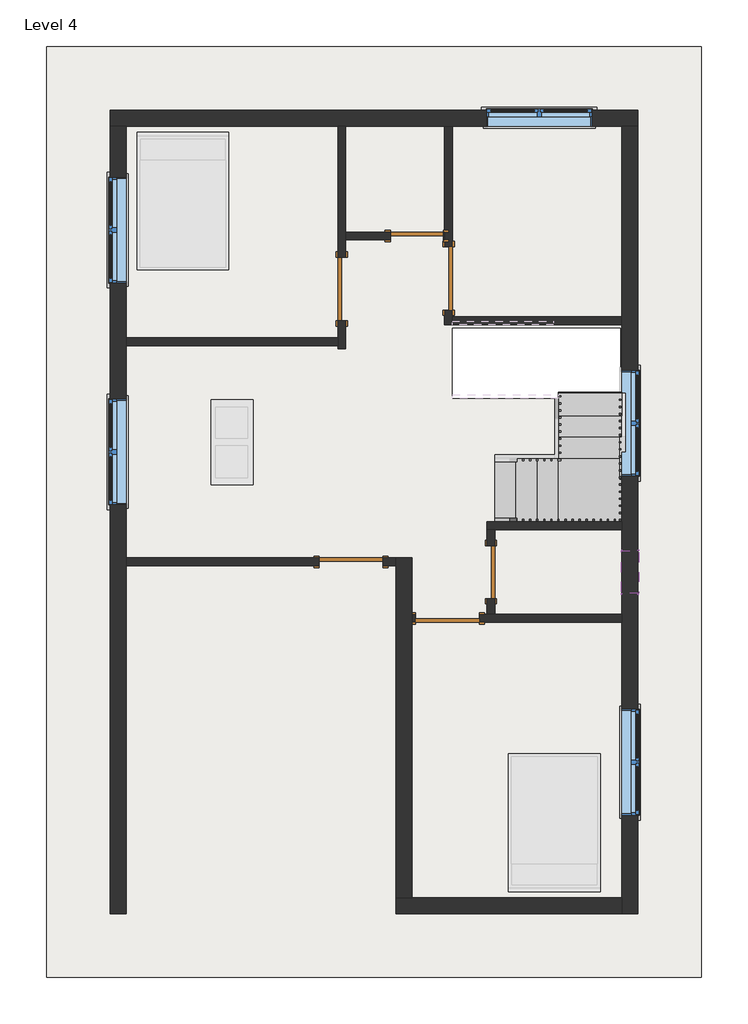
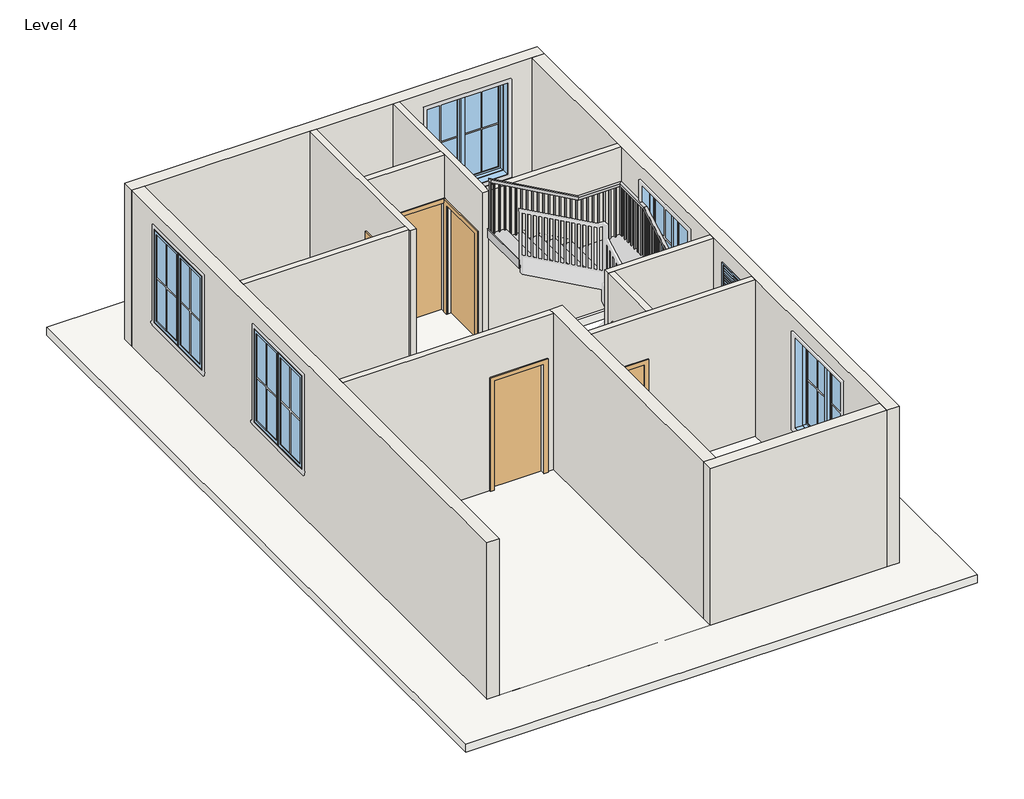
# One storey, part 1 of 2: 14 walls, 6 doors, 6 windows, 1 railing, 1 roof, 1 slab, 1 stair flight.
"""IFC4 building model written with IfcOpenShell, lengths in millimetres."""

from ifc_helpers import new_model, si_unit, frame, origin, place, context, project, spatial, polyline, outline, extrude, faceted_brep, transform, mapped, element, save
from components import door_214872d5, door_78caadf7, single_flush_door_3_e5f9f3c4, single_flush_door_3_305aa2a5, stair_flight_961aca31, window_casement_double_win_5_f93960c7, window_f2d8fef0

model = new_model("IFC4")

# Units and contexts
model_context = context("Model", 3, world=origin())
ifc_project = project(units=[si_unit("LENGTHUNIT", "METRE", prefix="MILLI")], contexts=[model_context])

# Site, building, storey
site = spatial("IfcSite", under=ifc_project)
building = spatial("IfcBuilding", under=site)
storey = spatial("IfcBuildingStorey", under=building, Name="Level 4", Elevation=6400.8)

# Doors
placement = place(None, origin())
door_shape = door_214872d5(model_context)
element("IfcDoor", 1, ObjectType="Single-Flush : DOOR 2'6\"", at=placement, inside=storey, context=model_context, shape_type="MappedRepresentation", body=[
    mapped(door_shape, transform((-185.4325206, 3926.3629493, 6400.8), x_axis=(1.0, 0.0, 0.0), y_axis=(0.0, 1.0, 0.0), z_axis=(0.0, 0.0, 1.0))),
])
door_2_shape = door_78caadf7(model_context)
element("IfcDoor", 2, ObjectType="Single-Flush : DOOR 2'6\"", at=placement, inside=storey, context=model_context, shape_type="MappedRepresentation", body=[
    mapped(door_2_shape, transform((881.3674794, -905.9870507, 6400.8), x_axis=(0.0, 1.0, 0.0), y_axis=(-1.0, 0.0, 0.0), z_axis=(0.0, 0.0, 1.0))),
])
single_flush_door_3_shape = single_flush_door_3_e5f9f3c4(model_context)
element("IfcDoor", 3, ObjectType="Single-Flush : DOOR 3'", at=placement, inside=storey, context=model_context, shape_type="MappedRepresentation", body=[
    mapped(single_flush_door_3_shape, transform((271.7674794, 3316.7629493, 6400.8), x_axis=(0.0, -1.0, 0.0), y_axis=(1.0, 0.0, 0.0), z_axis=(0.0, 0.0, 1.0))),
])
element("IfcDoor", 4, ObjectType="Single-Flush : DOOR 3'", at=placement, inside=storey, context=model_context, shape_type="MappedRepresentation", body=[
    mapped(single_flush_door_3_shape, transform((255.8924794, -1572.7370507, 6400.8), x_axis=(-1.0, 0.0, 0.0), y_axis=(0.0, -1.0, 0.0), z_axis=(0.0, 0.0, 1.0))),
])
single_flush_door_3_2_shape = single_flush_door_3_305aa2a5(model_context)
element("IfcDoor", 5, ObjectType="Single-Flush : DOOR 3'", at=placement, inside=storey, context=model_context, shape_type="MappedRepresentation", body=[
    mapped(single_flush_door_3_2_shape, transform((-1264.9325206, 3164.3629493, 6400.8), x_axis=(0.0, -1.0, 0.0), y_axis=(1.0, 0.0, 0.0), z_axis=(0.0, 0.0, 1.0))),
])
element("IfcDoor", 6, ObjectType="Single-Flush : DOOR 3'6\"", at=placement, inside=storey, context=model_context, shape_type="MappedRepresentation", body=[
    mapped(single_flush_door_3_shape, transform((-1131.5825206, -759.9370507, 6400.8), x_axis=(1.0, 0.0, 0.0), y_axis=(0.0, 1.0, 0.0), z_axis=(0.0, 0.0, 1.0))),
])

# Railing
element("IfcRailing", 7, ObjectType="Handrail - Rectangular", at=placement, inside=storey, context=model_context, shape_type="SolidModel", body=[
    faceted_brep([(938.5174794, -131.2870507, 7484.5333333), (938.5174794, -131.2870507, 7426.420221), (938.5174794, -182.0870507, 7426.420221), (938.5174794, -182.0870507, 7484.5333333), (2005.3174794, -131.2870507, 8077.2), (2018.4810817, -131.2870507, 8026.4), (2018.4810817, -182.0870507, 8026.4), (2005.3174794, -182.0870507, 8077.2), (2716.5174794, -131.2870507, 8077.2), (2716.5174794, -131.2870507, 8026.4), (2767.3174794, -182.0870507, 8026.4), (2767.3174794, -182.0870507, 8077.2), (2716.5174794, 579.9129493, 8077.2), (2716.5174794, 593.0765516, 8026.4), (2767.3174794, 593.0765516, 8026.4), (2767.3174794, 579.9129493, 8077.2), (2716.5174794, 1843.5629493, 8779.2277778), (2716.5174794, 1856.7265516, 8728.4277778), (2767.3174794, 1856.7265516, 8728.4277778), (2767.3174794, 1843.5629493, 8779.2277778), (2716.5174794, 2599.2129493, 8779.2277778), (2716.5174794, 2599.2129493, 8728.4277778), (2767.3174794, 2650.0129493, 8728.4277778), (2767.3174794, 2650.0129493, 8779.2277778), (1960.8674794, 2599.2129493, 8779.2277778), (1947.7038772, 2599.2129493, 8728.4277778), (1947.7038772, 2650.0129493, 8728.4277778), (1960.8674794, 2650.0129493, 8779.2277778), (328.9174794, 2599.2129493, 9685.8666667), (328.9174794, 2650.0129493, 9685.8666667), (328.9174794, 2650.0129493, 9627.7535543), (328.9174794, 2599.2129493, 9627.7535543)], [[[0, 1, 2, 3]], [[1, 0, 4, 5]], [[2, 1, 5, 6]], [[3, 2, 6, 7]], [[0, 3, 7, 4]], [[5, 4, 8, 9]], [[6, 5, 9, 10]], [[7, 6, 10, 11]], [[4, 7, 11, 8]], [[9, 8, 12, 13]], [[10, 9, 13, 14]], [[11, 10, 14, 15]], [[8, 11, 15, 12]], [[13, 12, 16, 17]], [[14, 13, 17, 18]], [[15, 14, 18, 19]], [[12, 15, 19, 16]], [[17, 16, 20, 21]], [[18, 17, 21, 22]], [[19, 18, 22, 23]], [[16, 19, 23, 20]], [[21, 20, 24, 25]], [[22, 21, 25, 26]], [[23, 22, 26, 27]], [[20, 23, 27, 24]], [[28, 29, 30, 31]], [[25, 24, 28, 31]], [[26, 25, 31, 30]], [[27, 26, 30, 29]], [[24, 27, 29, 28]]]),
    extrude(outline(polyline([(9580.1285543, 414.6424794), (9590.7118876, 395.5924794), (8602.1333333, 395.5924794), (8602.1333333, 414.6424794), (9580.1285543, 414.6424794)])), frame((0.0, 2615.0879493, 0.0), z_axis=(0.0, 1.0, 0.0), x_axis=(0.0, 0.0, 1.0)), (0.0, 0.0, 1.0), 19.05),
    extrude(outline(polyline([(9523.6841099, 516.2424794), (9534.2674432, 497.1924794), (8602.1333333, 497.1924794), (8602.1333333, 516.2424794), (9523.6841099, 516.2424794)])), frame((0.0, 2615.0879493, 0.0), z_axis=(0.0, 1.0, 0.0), x_axis=(0.0, 0.0, 1.0)), (0.0, 0.0, 1.0), 19.05),
    extrude(outline(polyline([(9467.2396654, 617.8424794), (9477.8229988, 598.7924794), (8602.1333333, 598.7924794), (8602.1333333, 617.8424794), (9467.2396654, 617.8424794)])), frame((0.0, 2615.0879493, 0.0), z_axis=(0.0, 1.0, 0.0), x_axis=(0.0, 0.0, 1.0)), (0.0, 0.0, 1.0), 19.05),
    extrude(outline(polyline([(9410.795221, 719.4424794), (9421.3785543, 700.3924794), (8432.8, 700.3924794), (8432.8, 719.4424794), (9410.795221, 719.4424794)])), frame((0.0, 2615.0879493, 0.0), z_axis=(0.0, 1.0, 0.0), x_axis=(0.0, 0.0, 1.0)), (0.0, 0.0, 1.0), 19.05),
    extrude(outline(polyline([(9354.3507765, 821.0424794), (9364.9341099, 801.9924794), (8432.8, 801.9924794), (8432.8, 821.0424794), (9354.3507765, 821.0424794)])), frame((0.0, 2615.0879493, 0.0), z_axis=(0.0, 1.0, 0.0), x_axis=(0.0, 0.0, 1.0)), (0.0, 0.0, 1.0), 19.05),
    extrude(outline(polyline([(9297.9063321, 922.6424794), (9308.4896654, 903.5924794), (8432.8, 903.5924794), (8432.8, 922.6424794), (9297.9063321, 922.6424794)])), frame((0.0, 2615.0879493, 0.0), z_axis=(0.0, 1.0, 0.0), x_axis=(0.0, 0.0, 1.0)), (0.0, 0.0, 1.0), 19.05),
    extrude(outline(polyline([(9241.4618876, 1024.2424794), (9252.045221, 1005.1924794), (8263.4666667, 1005.1924794), (8263.4666667, 1024.2424794), (9241.4618876, 1024.2424794)])), frame((0.0, 2615.0879493, 0.0), z_axis=(0.0, 1.0, 0.0), x_axis=(0.0, 0.0, 1.0)), (0.0, 0.0, 1.0), 19.05),
    extrude(outline(polyline([(9185.0174432, 1125.8424794), (9195.6007765, 1106.7924794), (8263.4666667, 1106.7924794), (8263.4666667, 1125.8424794), (9185.0174432, 1125.8424794)])), frame((0.0, 2615.0879493, 0.0), z_axis=(0.0, 1.0, 0.0), x_axis=(0.0, 0.0, 1.0)), (0.0, 0.0, 1.0), 19.05),
    extrude(outline(polyline([(9128.5729988, 1227.4424794), (9139.1563321, 1208.3924794), (8263.4666667, 1208.3924794), (8263.4666667, 1227.4424794), (9128.5729988, 1227.4424794)])), frame((0.0, 2615.0879493, 0.0), z_axis=(0.0, 1.0, 0.0), x_axis=(0.0, 0.0, 1.0)), (0.0, 0.0, 1.0), 19.05),
    extrude(outline(polyline([(9072.1285543, 1329.0424794), (9082.7118876, 1309.9924794), (8094.1333333, 1309.9924794), (8094.1333333, 1329.0424794), (9072.1285543, 1329.0424794)])), frame((0.0, 2615.0879493, 0.0), z_axis=(0.0, 1.0, 0.0), x_axis=(0.0, 0.0, 1.0)), (0.0, 0.0, 1.0), 19.05),
    extrude(outline(polyline([(9015.6841099, 1430.6424794), (9026.2674432, 1411.5924794), (8094.1333333, 1411.5924794), (8094.1333333, 1430.6424794), (9015.6841099, 1430.6424794)])), frame((0.0, 2615.0879493, 0.0), z_axis=(0.0, 1.0, 0.0), x_axis=(0.0, 0.0, 1.0)), (0.0, 0.0, 1.0), 19.05),
    extrude(outline(polyline([(8959.2396654, 1532.2424794), (8969.8229988, 1513.1924794), (8094.1333333, 1513.1924794), (8094.1333333, 1532.2424794), (8959.2396654, 1532.2424794)])), frame((0.0, 2615.0879493, 0.0), z_axis=(0.0, 1.0, 0.0), x_axis=(0.0, 0.0, 1.0)), (0.0, 0.0, 1.0), 19.05),
    extrude(outline(polyline([(8902.795221, 1633.8424794), (8913.3785543, 1614.7924794), (7924.8, 1614.7924794), (7924.8, 1633.8424794), (8902.795221, 1633.8424794)])), frame((0.0, 2615.0879493, 0.0), z_axis=(0.0, 1.0, 0.0), x_axis=(0.0, 0.0, 1.0)), (0.0, 0.0, 1.0), 19.05),
    extrude(outline(polyline([(8846.3507765, 1735.4424794), (8856.9341099, 1716.3924794), (7924.8, 1716.3924794), (7924.8, 1735.4424794), (8846.3507765, 1735.4424794)])), frame((0.0, 2615.0879493, 0.0), z_axis=(0.0, 1.0, 0.0), x_axis=(0.0, 0.0, 1.0)), (0.0, 0.0, 1.0), 19.05),
    extrude(outline(polyline([(8789.9063321, 1837.0424794), (8800.4896654, 1817.9924794), (7924.8, 1817.9924794), (7924.8, 1837.0424794), (8789.9063321, 1837.0424794)])), frame((0.0, 2615.0879493, 0.0), z_axis=(0.0, 1.0, 0.0), x_axis=(0.0, 0.0, 1.0)), (0.0, 0.0, 1.0), 19.05),
    extrude(outline(polyline([(8733.4618876, 1938.6424794), (8744.045221, 1919.5924794), (7755.4666667, 1919.5924794), (7755.4666667, 1938.6424794), (8733.4618876, 1938.6424794)])), frame((0.0, 2615.0879493, 0.0), z_axis=(0.0, 1.0, 0.0), x_axis=(0.0, 0.0, 1.0)), (0.0, 0.0, 1.0), 19.05),
    extrude(outline(polyline([(2040.2424794, 2634.1379493), (2040.2424794, 2615.0879493), (2021.1924794, 2615.0879493), (2021.1924794, 2634.1379493), (2040.2424794, 2634.1379493)])), frame((0.0, 0.0, 7755.4666667), z_axis=(0.0, 0.0, 1.0), x_axis=(1.0, 0.0, 0.0)), (0.0, 0.0, 1.0), 972.9611111),
    extrude(outline(polyline([(2141.8424794, 2634.1379493), (2141.8424794, 2615.0879493), (2122.7924794, 2615.0879493), (2122.7924794, 2634.1379493), (2141.8424794, 2634.1379493)])), frame((0.0, 0.0, 7755.4666667), z_axis=(0.0, 0.0, 1.0), x_axis=(1.0, 0.0, 0.0)), (0.0, 0.0, 1.0), 972.9611111),
    extrude(outline(polyline([(2243.4424794, 2634.1379493), (2243.4424794, 2615.0879493), (2224.3924794, 2615.0879493), (2224.3924794, 2634.1379493), (2243.4424794, 2634.1379493)])), frame((0.0, 0.0, 7755.4666667), z_axis=(0.0, 0.0, 1.0), x_axis=(1.0, 0.0, 0.0)), (0.0, 0.0, 1.0), 972.9611111),
    extrude(outline(polyline([(2345.0424794, 2634.1379493), (2345.0424794, 2615.0879493), (2325.9924794, 2615.0879493), (2325.9924794, 2634.1379493), (2345.0424794, 2634.1379493)])), frame((0.0, 0.0, 7755.4666667), z_axis=(0.0, 0.0, 1.0), x_axis=(1.0, 0.0, 0.0)), (0.0, 0.0, 1.0), 972.9611111),
    extrude(outline(polyline([(2446.6424794, 2634.1379493), (2446.6424794, 2615.0879493), (2427.5924794, 2615.0879493), (2427.5924794, 2634.1379493), (2446.6424794, 2634.1379493)])), frame((0.0, 0.0, 7755.4666667), z_axis=(0.0, 0.0, 1.0), x_axis=(1.0, 0.0, 0.0)), (0.0, 0.0, 1.0), 972.9611111),
    extrude(outline(polyline([(2548.2424794, 2634.1379493), (2548.2424794, 2615.0879493), (2529.1924794, 2615.0879493), (2529.1924794, 2634.1379493), (2548.2424794, 2634.1379493)])), frame((0.0, 0.0, 7755.4666667), z_axis=(0.0, 0.0, 1.0), x_axis=(1.0, 0.0, 0.0)), (0.0, 0.0, 1.0), 972.9611111),
    extrude(outline(polyline([(2649.8424794, 2634.1379493), (2649.8424794, 2615.0879493), (2630.7924794, 2615.0879493), (2630.7924794, 2634.1379493), (2649.8424794, 2634.1379493)])), frame((0.0, 0.0, 7755.4666667), z_axis=(0.0, 0.0, 1.0), x_axis=(1.0, 0.0, 0.0)), (0.0, 0.0, 1.0), 972.9611111),
    extrude(outline(polyline([(2751.4424794, 2576.9879493), (2732.3924794, 2576.9879493), (2732.3924794, 2596.0379493), (2751.4424794, 2596.0379493), (2751.4424794, 2576.9879493)])), frame((0.0, 0.0, 7755.4666667), z_axis=(0.0, 0.0, 1.0), x_axis=(1.0, 0.0, 0.0)), (0.0, 0.0, 1.0), 972.9611111),
    extrude(outline(polyline([(2751.4424794, 2475.3879493), (2732.3924794, 2475.3879493), (2732.3924794, 2494.4379493), (2751.4424794, 2494.4379493), (2751.4424794, 2475.3879493)])), frame((0.0, 0.0, 7755.4666667), z_axis=(0.0, 0.0, 1.0), x_axis=(1.0, 0.0, 0.0)), (0.0, 0.0, 1.0), 972.9611111),
    extrude(outline(polyline([(2751.4424794, 2373.7879493), (2732.3924794, 2373.7879493), (2732.3924794, 2392.8379493), (2751.4424794, 2392.8379493), (2751.4424794, 2373.7879493)])), frame((0.0, 0.0, 7755.4666667), z_axis=(0.0, 0.0, 1.0), x_axis=(1.0, 0.0, 0.0)), (0.0, 0.0, 1.0), 972.9611111),
    extrude(outline(polyline([(2751.4424794, 2272.1879493), (2732.3924794, 2272.1879493), (2732.3924794, 2291.2379493), (2751.4424794, 2291.2379493), (2751.4424794, 2272.1879493)])), frame((0.0, 0.0, 7755.4666667), z_axis=(0.0, 0.0, 1.0), x_axis=(1.0, 0.0, 0.0)), (0.0, 0.0, 1.0), 972.9611111),
    extrude(outline(polyline([(2751.4424794, 2170.5879493), (2732.3924794, 2170.5879493), (2732.3924794, 2189.6379493), (2751.4424794, 2189.6379493), (2751.4424794, 2170.5879493)])), frame((0.0, 0.0, 7755.4666667), z_axis=(0.0, 0.0, 1.0), x_axis=(1.0, 0.0, 0.0)), (0.0, 0.0, 1.0), 972.9611111),
    extrude(outline(polyline([(2751.4424794, 2068.9879493), (2732.3924794, 2068.9879493), (2732.3924794, 2088.0379493), (2751.4424794, 2088.0379493), (2751.4424794, 2068.9879493)])), frame((0.0, 0.0, 7755.4666667), z_axis=(0.0, 0.0, 1.0), x_axis=(1.0, 0.0, 0.0)), (0.0, 0.0, 1.0), 972.9611111),
    extrude(outline(polyline([(2751.4424794, 1967.3879493), (2732.3924794, 1967.3879493), (2732.3924794, 1986.4379493), (2751.4424794, 1986.4379493), (2751.4424794, 1967.3879493)])), frame((0.0, 0.0, 7755.4666667), z_axis=(0.0, 0.0, 1.0), x_axis=(1.0, 0.0, 0.0)), (0.0, 0.0, 1.0), 972.9611111),
    extrude(outline(polyline([(2751.4424794, 1865.7879493), (2732.3924794, 1865.7879493), (2732.3924794, 1884.8379493), (2751.4424794, 1884.8379493), (2751.4424794, 1865.7879493)])), frame((0.0, 0.0, 7755.4666667), z_axis=(0.0, 0.0, 1.0), x_axis=(1.0, 0.0, 0.0)), (0.0, 0.0, 1.0), 972.9611111),
    extrude(outline(polyline([(1764.1879493, 8677.0174432), (1783.2379493, 8687.6007765), (1783.2379493, 7755.4666667), (1764.1879493, 7755.4666667), (1764.1879493, 8677.0174432)])), frame((2732.3924794, 0.0, 0.0), z_axis=(1.0, 0.0, 0.0), x_axis=(0.0, 1.0, 0.0)), (0.0, 0.0, 1.0), 19.05),
    extrude(outline(polyline([(1662.5879493, 8620.5729988), (1681.6379493, 8631.1563321), (1681.6379493, 7755.4666667), (1662.5879493, 7755.4666667), (1662.5879493, 8620.5729988)])), frame((2732.3924794, 0.0, 0.0), z_axis=(1.0, 0.0, 0.0), x_axis=(0.0, 1.0, 0.0)), (0.0, 0.0, 1.0), 19.05),
    extrude(outline(polyline([(1560.9879493, 8564.1285543), (1580.0379493, 8574.7118876), (1580.0379493, 7586.1333333), (1560.9879493, 7586.1333333), (1560.9879493, 8564.1285543)])), frame((2732.3924794, 0.0, 0.0), z_axis=(1.0, 0.0, 0.0), x_axis=(0.0, 1.0, 0.0)), (0.0, 0.0, 1.0), 19.05),
    extrude(outline(polyline([(1459.3879493, 8507.6841099), (1478.4379493, 8518.2674432), (1478.4379493, 7586.1333333), (1459.3879493, 7586.1333333), (1459.3879493, 8507.6841099)])), frame((2732.3924794, 0.0, 0.0), z_axis=(1.0, 0.0, 0.0), x_axis=(0.0, 1.0, 0.0)), (0.0, 0.0, 1.0), 19.05),
    extrude(outline(polyline([(1357.7879493, 8451.2396654), (1376.8379493, 8461.8229988), (1376.8379493, 7586.1333333), (1357.7879493, 7586.1333333), (1357.7879493, 8451.2396654)])), frame((2732.3924794, 0.0, 0.0), z_axis=(1.0, 0.0, 0.0), x_axis=(0.0, 1.0, 0.0)), (0.0, 0.0, 1.0), 19.05),
    extrude(outline(polyline([(1256.1879493, 8394.795221), (1275.2379493, 8405.3785543), (1275.2379493, 7416.8), (1256.1879493, 7416.8), (1256.1879493, 8394.795221)])), frame((2732.3924794, 0.0, 0.0), z_axis=(1.0, 0.0, 0.0), x_axis=(0.0, 1.0, 0.0)), (0.0, 0.0, 1.0), 19.05),
    extrude(outline(polyline([(1154.5879493, 8338.3507765), (1173.6379493, 8348.9341099), (1173.6379493, 7416.8), (1154.5879493, 7416.8), (1154.5879493, 8338.3507765)])), frame((2732.3924794, 0.0, 0.0), z_axis=(1.0, 0.0, 0.0), x_axis=(0.0, 1.0, 0.0)), (0.0, 0.0, 1.0), 19.05),
    extrude(outline(polyline([(1052.9879493, 8281.9063321), (1072.0379493, 8292.4896654), (1072.0379493, 7416.8), (1052.9879493, 7416.8), (1052.9879493, 8281.9063321)])), frame((2732.3924794, 0.0, 0.0), z_axis=(1.0, 0.0, 0.0), x_axis=(0.0, 1.0, 0.0)), (0.0, 0.0, 1.0), 19.05),
    extrude(outline(polyline([(951.3879493, 8225.4618876), (970.4379493, 8236.045221), (970.4379493, 7247.4666667), (951.3879493, 7247.4666667), (951.3879493, 8225.4618876)])), frame((2732.3924794, 0.0, 0.0), z_axis=(1.0, 0.0, 0.0), x_axis=(0.0, 1.0, 0.0)), (0.0, 0.0, 1.0), 19.05),
    extrude(outline(polyline([(849.7879493, 8169.0174432), (868.8379493, 8179.6007765), (868.8379493, 7247.4666667), (849.7879493, 7247.4666667), (849.7879493, 8169.0174432)])), frame((2732.3924794, 0.0, 0.0), z_axis=(1.0, 0.0, 0.0), x_axis=(0.0, 1.0, 0.0)), (0.0, 0.0, 1.0), 19.05),
    extrude(outline(polyline([(748.1879493, 8112.5729988), (767.2379493, 8123.1563321), (767.2379493, 7247.4666667), (748.1879493, 7247.4666667), (748.1879493, 8112.5729988)])), frame((2732.3924794, 0.0, 0.0), z_axis=(1.0, 0.0, 0.0), x_axis=(0.0, 1.0, 0.0)), (0.0, 0.0, 1.0), 19.05),
    extrude(outline(polyline([(646.5879493, 8056.1285543), (665.6379493, 8066.7118876), (665.6379493, 7078.1333333), (646.5879493, 7078.1333333), (646.5879493, 8056.1285543)])), frame((2732.3924794, 0.0, 0.0), z_axis=(1.0, 0.0, 0.0), x_axis=(0.0, 1.0, 0.0)), (0.0, 0.0, 1.0), 19.05),
    extrude(outline(polyline([(2751.4424794, 544.9879493), (2732.3924794, 544.9879493), (2732.3924794, 564.0379493), (2751.4424794, 564.0379493), (2751.4424794, 544.9879493)])), frame((0.0, 0.0, 7078.1333333), z_axis=(0.0, 0.0, 1.0), x_axis=(1.0, 0.0, 0.0)), (0.0, 0.0, 1.0), 948.2666667),
    extrude(outline(polyline([(2751.4424794, 443.3879493), (2732.3924794, 443.3879493), (2732.3924794, 462.4379493), (2751.4424794, 462.4379493), (2751.4424794, 443.3879493)])), frame((0.0, 0.0, 7078.1333333), z_axis=(0.0, 0.0, 1.0), x_axis=(1.0, 0.0, 0.0)), (0.0, 0.0, 1.0), 948.2666667),
    extrude(outline(polyline([(2751.4424794, 341.7879493), (2732.3924794, 341.7879493), (2732.3924794, 360.8379493), (2751.4424794, 360.8379493), (2751.4424794, 341.7879493)])), frame((0.0, 0.0, 7078.1333333), z_axis=(0.0, 0.0, 1.0), x_axis=(1.0, 0.0, 0.0)), (0.0, 0.0, 1.0), 948.2666667),
    extrude(outline(polyline([(2751.4424794, 240.1879493), (2732.3924794, 240.1879493), (2732.3924794, 259.2379493), (2751.4424794, 259.2379493), (2751.4424794, 240.1879493)])), frame((0.0, 0.0, 7078.1333333), z_axis=(0.0, 0.0, 1.0), x_axis=(1.0, 0.0, 0.0)), (0.0, 0.0, 1.0), 948.2666667),
    extrude(outline(polyline([(2751.4424794, 138.5879493), (2732.3924794, 138.5879493), (2732.3924794, 157.6379493), (2751.4424794, 157.6379493), (2751.4424794, 138.5879493)])), frame((0.0, 0.0, 7078.1333333), z_axis=(0.0, 0.0, 1.0), x_axis=(1.0, 0.0, 0.0)), (0.0, 0.0, 1.0), 948.2666667),
    extrude(outline(polyline([(2751.4424794, 36.9879493), (2732.3924794, 36.9879493), (2732.3924794, 56.0379493), (2751.4424794, 56.0379493), (2751.4424794, 36.9879493)])), frame((0.0, 0.0, 7078.1333333), z_axis=(0.0, 0.0, 1.0), x_axis=(1.0, 0.0, 0.0)), (0.0, 0.0, 1.0), 948.2666667),
    extrude(outline(polyline([(2751.4424794, -64.6120507), (2732.3924794, -64.6120507), (2732.3924794, -45.5620507), (2751.4424794, -45.5620507), (2751.4424794, -64.6120507)])), frame((0.0, 0.0, 7078.1333333), z_axis=(0.0, 0.0, 1.0), x_axis=(1.0, 0.0, 0.0)), (0.0, 0.0, 1.0), 948.2666667),
    extrude(outline(polyline([(2656.1924794, -166.2120507), (2656.1924794, -147.1620507), (2675.2424794, -147.1620507), (2675.2424794, -166.2120507), (2656.1924794, -166.2120507)])), frame((0.0, 0.0, 7078.1333333), z_axis=(0.0, 0.0, 1.0), x_axis=(1.0, 0.0, 0.0)), (0.0, 0.0, 1.0), 948.2666667),
    extrude(outline(polyline([(2554.5924794, -166.2120507), (2554.5924794, -147.1620507), (2573.6424794, -147.1620507), (2573.6424794, -166.2120507), (2554.5924794, -166.2120507)])), frame((0.0, 0.0, 7078.1333333), z_axis=(0.0, 0.0, 1.0), x_axis=(1.0, 0.0, 0.0)), (0.0, 0.0, 1.0), 948.2666667),
    extrude(outline(polyline([(2452.9924794, -166.2120507), (2452.9924794, -147.1620507), (2472.0424794, -147.1620507), (2472.0424794, -166.2120507), (2452.9924794, -166.2120507)])), frame((0.0, 0.0, 7078.1333333), z_axis=(0.0, 0.0, 1.0), x_axis=(1.0, 0.0, 0.0)), (0.0, 0.0, 1.0), 948.2666667),
    extrude(outline(polyline([(2351.3924794, -166.2120507), (2351.3924794, -147.1620507), (2370.4424794, -147.1620507), (2370.4424794, -166.2120507), (2351.3924794, -166.2120507)])), frame((0.0, 0.0, 7078.1333333), z_axis=(0.0, 0.0, 1.0), x_axis=(1.0, 0.0, 0.0)), (0.0, 0.0, 1.0), 948.2666667),
    extrude(outline(polyline([(2249.7924794, -166.2120507), (2249.7924794, -147.1620507), (2268.8424794, -147.1620507), (2268.8424794, -166.2120507), (2249.7924794, -166.2120507)])), frame((0.0, 0.0, 7078.1333333), z_axis=(0.0, 0.0, 1.0), x_axis=(1.0, 0.0, 0.0)), (0.0, 0.0, 1.0), 948.2666667),
    extrude(outline(polyline([(2148.1924794, -166.2120507), (2148.1924794, -147.1620507), (2167.2424794, -147.1620507), (2167.2424794, -166.2120507), (2148.1924794, -166.2120507)])), frame((0.0, 0.0, 7078.1333333), z_axis=(0.0, 0.0, 1.0), x_axis=(1.0, 0.0, 0.0)), (0.0, 0.0, 1.0), 948.2666667),
    extrude(outline(polyline([(2046.5924794, -166.2120507), (2046.5924794, -147.1620507), (2065.6424794, -147.1620507), (2065.6424794, -166.2120507), (2046.5924794, -166.2120507)])), frame((0.0, 0.0, 7078.1333333), z_axis=(0.0, 0.0, 1.0), x_axis=(1.0, 0.0, 0.0)), (0.0, 0.0, 1.0), 948.2666667),
    extrude(outline(polyline([(7996.1563321, 1964.0424794), (7985.5729988, 1944.9924794), (7078.1333333, 1944.9924794), (7078.1333333, 1964.0424794), (7996.1563321, 1964.0424794)])), frame((0.0, -166.2120507, 0.0), z_axis=(0.0, 1.0, 0.0), x_axis=(0.0, 0.0, 1.0)), (0.0, 0.0, 1.0), 19.05),
    extrude(outline(polyline([(7939.7118876, 1862.4424794), (7929.1285543, 1843.3924794), (7078.1333333, 1843.3924794), (7078.1333333, 1862.4424794), (7939.7118876, 1862.4424794)])), frame((0.0, -166.2120507, 0.0), z_axis=(0.0, 1.0, 0.0), x_axis=(0.0, 0.0, 1.0)), (0.0, 0.0, 1.0), 19.05),
    extrude(outline(polyline([(7883.2674432, 1760.8424794), (7872.6841099, 1741.7924794), (6908.8, 1741.7924794), (6908.8, 1760.8424794), (7883.2674432, 1760.8424794)])), frame((0.0, -166.2120507, 0.0), z_axis=(0.0, 1.0, 0.0), x_axis=(0.0, 0.0, 1.0)), (0.0, 0.0, 1.0), 19.05),
    extrude(outline(polyline([(7826.8229988, 1659.2424794), (7816.2396654, 1640.1924794), (6908.8, 1640.1924794), (6908.8, 1659.2424794), (7826.8229988, 1659.2424794)])), frame((0.0, -166.2120507, 0.0), z_axis=(0.0, 1.0, 0.0), x_axis=(0.0, 0.0, 1.0)), (0.0, 0.0, 1.0), 19.05),
    extrude(outline(polyline([(7770.3785543, 1557.6424794), (7759.795221, 1538.5924794), (6908.8, 1538.5924794), (6908.8, 1557.6424794), (7770.3785543, 1557.6424794)])), frame((0.0, -166.2120507, 0.0), z_axis=(0.0, 1.0, 0.0), x_axis=(0.0, 0.0, 1.0)), (0.0, 0.0, 1.0), 19.05),
    extrude(outline(polyline([(7713.9341099, 1456.0424794), (7703.3507765, 1436.9924794), (6739.4666667, 1436.9924794), (6739.4666667, 1456.0424794), (7713.9341099, 1456.0424794)])), frame((0.0, -166.2120507, 0.0), z_axis=(0.0, 1.0, 0.0), x_axis=(0.0, 0.0, 1.0)), (0.0, 0.0, 1.0), 19.05),
    extrude(outline(polyline([(7657.4896654, 1354.4424794), (7646.9063321, 1335.3924794), (6739.4666667, 1335.3924794), (6739.4666667, 1354.4424794), (7657.4896654, 1354.4424794)])), frame((0.0, -166.2120507, 0.0), z_axis=(0.0, 1.0, 0.0), x_axis=(0.0, 0.0, 1.0)), (0.0, 0.0, 1.0), 19.05),
    extrude(outline(polyline([(7601.045221, 1252.8424794), (7590.4618876, 1233.7924794), (6739.4666667, 1233.7924794), (6739.4666667, 1252.8424794), (7601.045221, 1252.8424794)])), frame((0.0, -166.2120507, 0.0), z_axis=(0.0, 1.0, 0.0), x_axis=(0.0, 0.0, 1.0)), (0.0, 0.0, 1.0), 19.05),
    extrude(outline(polyline([(7544.6007765, 1151.2424794), (7534.0174432, 1132.1924794), (6570.1333333, 1132.1924794), (6570.1333333, 1151.2424794), (7544.6007765, 1151.2424794)])), frame((0.0, -166.2120507, 0.0), z_axis=(0.0, 1.0, 0.0), x_axis=(0.0, 0.0, 1.0)), (0.0, 0.0, 1.0), 19.05),
    extrude(outline(polyline([(7488.1563321, 1049.6424794), (7477.5729988, 1030.5924794), (6570.1333333, 1030.5924794), (6570.1333333, 1049.6424794), (7488.1563321, 1049.6424794)])), frame((0.0, -166.2120507, 0.0), z_axis=(0.0, 1.0, 0.0), x_axis=(0.0, 0.0, 1.0)), (0.0, 0.0, 1.0), 19.05),
    extrude(outline(polyline([(2751.4424794, 2615.0879493), (2732.3924794, 2615.0879493), (2732.3924794, 2634.1379493), (2751.4424794, 2634.1379493), (2751.4424794, 2615.0879493)])), frame((0.0, 0.0, 7755.4666667), z_axis=(0.0, 0.0, 1.0), x_axis=(1.0, 0.0, 0.0)), (0.0, 0.0, 1.0), 972.9611111),
    extrude(outline(polyline([(2732.3924794, -166.2120507), (2732.3924794, -147.1620507), (2751.4424794, -147.1620507), (2751.4424794, -166.2120507), (2732.3924794, -166.2120507)])), frame((0.0, 0.0, 7078.1333333), z_axis=(0.0, 0.0, 1.0), x_axis=(1.0, 0.0, 0.0)), (0.0, 0.0, 1.0), 948.2666667),
    extrude(outline(polyline([(9617.170221, 347.9674794), (9627.7535543, 328.9174794), (8602.1333333, 328.9174794), (8602.1333333, 347.9674794), (9617.170221, 347.9674794)])), frame((0.0, 2615.0879493, 0.0), z_axis=(0.0, 1.0, 0.0), x_axis=(0.0, 0.0, 1.0)), (0.0, 0.0, 1.0), 19.05),
    extrude(outline(polyline([(7437.0035543, 957.5674794), (7426.420221, 938.5174794), (6570.1333333, 938.5174794), (6570.1333333, 957.5674794), (7437.0035543, 957.5674794)])), frame((0.0, -166.2120507, 0.0), z_axis=(0.0, 1.0, 0.0), x_axis=(0.0, 0.0, 1.0)), (0.0, 0.0, 1.0), 19.05),
])

# Roof
element("IfcRoof", 8, ObjectType="ROOF 6\"", at=placement, inside=storey, context=model_context, shape_type="SweptSolid", body=[
    extrude(outline(polyline([(-5513.0825206, 6650.5129493), (3910.3174794, 6650.5129493), (3910.3174794, -6735.2870507), (-5513.0825206, -6735.2870507), (-5513.0825206, 6650.5129493)]), holes=[polyline([(2741.9174794, -156.6870507), (2741.9174794, 2599.2129493), (328.9174794, 2599.2129493), (328.9174794, 1595.9129493), (1802.1174794, 1595.9129493), (1802.1174794, 706.9129493), (1040.1174794, 706.9129493), (1040.1174794, -156.6870507), (2741.9174794, -156.6870507)])]), frame((0.0, 0.0, 6248.4), z_axis=(0.0, 0.0, 1.0), x_axis=(1.0, 0.0, 0.0)), (0.0, 0.0, 1.0), 152.4),
])

# Slab
element("IfcSlab", 9, ObjectType="FLOOR 6\"", at=placement, inside=storey, context=model_context, shape_type="SweptSolid", body=[
    extrude(outline(polyline([(2995.9174794, 5736.1129493), (2995.9174794, -5820.8870507), (-4598.6825206, -5820.8870507), (-4598.6825206, 5736.1129493), (2995.9174794, 5736.1129493)]), holes=[polyline([(2741.9174794, -156.6870507), (2741.9174794, 2599.2129493), (328.9174794, 2599.2129493), (328.9174794, 1595.9129493), (1802.1174794, 1595.9129493), (1802.1174794, 706.9129493), (1040.1174794, 706.9129493), (1040.1174794, -156.6870507), (2741.9174794, -156.6870507)])]), frame((0.0, 0.0, 6248.4), z_axis=(0.0, 0.0, 1.0), x_axis=(1.0, 0.0, 0.0)), (0.0, 0.0, 1.0), 152.4),
])

# Stair flight
stair_flight_shape = stair_flight_961aca31(model_context)
element("IfcStairFlight", 10, ObjectType="2\" Tread 1\" Nosing 1/4\" Riser", at=placement, inside=storey, context=model_context, shape_type="MappedRepresentation", body=[
    mapped(stair_flight_shape, transform((0.0, 0.0, 0.0), x_axis=(1.0, 0.0, 0.0), y_axis=(0.0, 1.0, 0.0), z_axis=(0.0, 0.0, 1.0))),
])

# Walls
element("IfcWall", 11, at=placement, inside=storey, context=model_context, shape_type="Brep", body=[
    faceted_brep([(-1322.0825206, 2707.1629493, 8534.4), (-1322.0825206, 2707.1629493, 6400.8), (-1322.0825206, 2459.5129493, 6400.8), (-1322.0825206, 2345.2129493, 6400.8), (-1322.0825206, 2307.1129493, 6400.8), (-1322.0825206, 2307.1129493, 9448.8), (-1322.0825206, 2345.2129493, 9448.8), (-1322.0825206, 2459.5129493, 9448.8), (-1322.0825206, 5507.5129493, 9448.8), (-1322.0825206, 5507.5129493, 6400.8), (-1322.0825206, 3621.5629493, 6400.8), (-1322.0825206, 3621.5629493, 8534.4), (-1207.7825206, 2307.1129493, 6400.8), (-1207.7825206, 2707.1629493, 6400.8), (-1207.7825206, 2707.1629493, 8534.4), (-1207.7825206, 3621.5629493, 8534.4), (-1207.7825206, 3621.5629493, 6400.8), (-1207.7825206, 3869.2129493, 6400.8), (-1207.7825206, 3983.5129493, 6400.8), (-1207.7825206, 5507.5129493, 6400.8), (-1207.7825206, 5507.5129493, 9448.8), (-1207.7825206, 3983.5129493, 9448.8), (-1207.7825206, 3869.2129493, 9448.8), (-1207.7825206, 2307.1129493, 9448.8)], [[[0, 1, 2, 3, 4, 5, 6, 7, 8, 9, 10, 11]], [[12, 13, 14, 15, 16, 17, 18, 19, 20, 21, 22, 23]], [[10, 9, 19, 18, 17, 16]], [[4, 3, 2, 1, 13, 12]], [[5, 4, 12, 23]], [[9, 8, 20, 19]], [[14, 13, 1, 0]], [[15, 14, 0, 11]], [[16, 15, 11, 10]], [[8, 7, 6, 5, 23, 22, 21, 20]]]),
])
element("IfcWall", 12, at=placement, inside=storey, context=model_context, shape_type="SweptSolid", body=[
    extrude(outline(polyline([(-1322.0825206, 2345.2129493), (-4370.0825206, 2345.2129493), (-4370.0825206, 2459.5129493), (-1322.0825206, 2459.5129493), (-1322.0825206, 2345.2129493)])), frame((0.0, 0.0, 6400.8), z_axis=(0.0, 0.0, 1.0), x_axis=(1.0, 0.0, 0.0)), (0.0, 0.0, 1.0), 3048.0),
])
element("IfcWall", 13, at=placement, inside=storey, context=model_context, shape_type="SweptSolid", body=[
    extrude(outline(polyline([(8534.4, 195.5674794), (6400.8, 195.5674794), (6400.8, 214.6174794), (9448.8, 214.6174794), (9448.8, -1207.7825206), (6400.8, -1207.7825206), (6400.8, -566.4325206), (8534.4, -566.4325206), (8534.4, 195.5674794)])), frame((0.0, 3869.2129493, 0.0), z_axis=(0.0, 1.0, 0.0), x_axis=(0.0, 0.0, 1.0)), (0.0, 0.0, 1.0), 114.3),
])
element("IfcWall", 14, at=placement, inside=storey, context=model_context, shape_type="Brep", body=[
    faceted_brep([(214.6174794, 2859.5629493, 8534.4), (214.6174794, 2859.5629493, 6400.8), (214.6174794, 2650.0129493, 6400.8), (214.6174794, 2650.0129493, 9448.8), (214.6174794, 3869.2129493, 9448.8), (214.6174794, 3983.5129493, 9448.8), (214.6174794, 5507.5129493, 9448.8), (214.6174794, 5507.5129493, 6400.8), (214.6174794, 3983.5129493, 6400.8), (214.6174794, 3869.2129493, 6400.8), (214.6174794, 3773.9629493, 6400.8), (214.6174794, 3773.9629493, 8534.4), (328.9174794, 2650.0129493, 6400.8), (328.9174794, 2764.3129493, 6400.8), (328.9174794, 2859.5629493, 6400.8), (328.9174794, 2859.5629493, 8534.4), (328.9174794, 3773.9629493, 8534.4), (328.9174794, 3773.9629493, 6400.8), (328.9174794, 5507.5129493, 6400.8), (328.9174794, 5507.5129493, 9448.8), (328.9174794, 2764.3129493, 9448.8), (328.9174794, 2650.0129493, 9448.8)], [[[0, 1, 2, 3, 4, 5, 6, 7, 8, 9, 10, 11]], [[12, 13, 14, 15, 16, 17, 18, 19, 20, 21]], [[2, 1, 14, 13, 12]], [[10, 9, 8, 7, 18, 17]], [[7, 6, 19, 18]], [[3, 2, 12, 21]], [[15, 14, 1, 0]], [[16, 15, 0, 11]], [[17, 16, 11, 10]], [[6, 5, 4, 3, 21, 20, 19]]]),
])
element("IfcWall", 15, at=placement, inside=storey, context=model_context, shape_type="SweptSolid", body=[
    extrude(outline(polyline([(2767.3174794, 2650.0129493), (328.9174794, 2650.0129493), (328.9174794, 2764.3129493), (2767.3174794, 2764.3129493), (2767.3174794, 2650.0129493)])), frame((0.0, 0.0, 6400.8), z_axis=(0.0, 0.0, 1.0), x_axis=(1.0, 0.0, 0.0)), (0.0, 0.0, 1.0), 3048.0),
])
element("IfcWall", 16, at=placement, inside=storey, context=model_context, shape_type="Brep", body=[
    faceted_brep([(2767.3174794, -182.0870507, 6400.8), (824.2174794, -182.0870507, 6400.8), (824.2174794, -182.0870507, 9448.8), (2767.3174794, -182.0870507, 9448.8), (2767.3174794, -296.3870507, 6400.8), (2767.3174794, -296.3870507, 9448.8), (938.5174794, -296.3870507, 9448.8), (824.2174794, -296.3870507, 9448.8), (824.2174794, -296.3870507, 6400.8), (938.5174794, -296.3870507, 6400.8)], [[[0, 1, 2, 3]], [[4, 5, 6, 7, 8, 9]], [[1, 0, 4, 9, 8]], [[0, 3, 5, 4]], [[2, 1, 8, 7]], [[3, 2, 7, 6, 5]]]),
])
element("IfcWall", 17, at=placement, inside=storey, context=model_context, shape_type="SweptSolid", body=[
    extrude(outline(polyline([(-296.3870507, 6400.8), (-524.9870507, 6400.8), (-524.9870507, 8534.4), (-1286.9870507, 8534.4), (-1286.9870507, 6400.8), (-1515.5870507, 6400.8), (-1515.5870507, 9448.8), (-296.3870507, 9448.8), (-296.3870507, 6400.8)])), frame((824.2174794, 0.0, 0.0), z_axis=(1.0, 0.0, 0.0), x_axis=(0.0, 1.0, 0.0)), (0.0, 0.0, 1.0), 114.3),
])
element("IfcWall", 18, at=placement, inside=storey, context=model_context, shape_type="Brep", body=[
    faceted_brep([(-201.3075206, -1515.5870507, 8534.4), (-201.3075206, -1515.5870507, 6400.8), (-255.2825206, -1515.5870507, 6400.8), (-255.2825206, -1515.5870507, 9448.8), (824.2174794, -1515.5870507, 9448.8), (938.5174794, -1515.5870507, 9448.8), (2767.3174794, -1515.5870507, 9448.8), (2767.3174794, -1515.5870507, 6400.8), (938.5174794, -1515.5870507, 6400.8), (824.2174794, -1515.5870507, 6400.8), (713.0924794, -1515.5870507, 6400.8), (713.0924794, -1515.5870507, 8534.4), (-255.2825206, -1629.8870507, 6400.8), (-201.3075206, -1629.8870507, 6400.8), (-201.3075206, -1629.8870507, 8534.4), (713.0924794, -1629.8870507, 8534.4), (713.0924794, -1629.8870507, 6400.8), (2767.3174794, -1629.8870507, 6400.8), (2767.3174794, -1629.8870507, 9448.8), (-255.2825206, -1629.8870507, 9448.8)], [[[0, 1, 2, 3, 4, 5, 6, 7, 8, 9, 10, 11]], [[12, 13, 14, 15, 16, 17, 18, 19]], [[2, 1, 13, 12]], [[10, 9, 8, 7, 17, 16]], [[7, 6, 18, 17]], [[3, 2, 12, 19]], [[14, 13, 1, 0]], [[15, 14, 0, 11]], [[16, 15, 11, 10]], [[6, 5, 4, 3, 19, 18]]]),
])
element("IfcWall", 19, at=placement, inside=storey, context=model_context, shape_type="SweptSolid", body=[
    extrude(outline(polyline([(8534.4, -674.3825206), (6400.8, -674.3825206), (6400.8, -483.8825206), (9448.8, -483.8825206), (9448.8, -4370.0825206), (6400.8, -4370.0825206), (6400.8, -1588.7825206), (8534.4, -1588.7825206), (8534.4, -674.3825206)])), frame((0.0, -817.0870507, 0.0), z_axis=(0.0, 1.0, 0.0), x_axis=(0.0, 0.0, 1.0)), (0.0, 0.0, 1.0), 114.3),
])
element("IfcWall", 20, ObjectType="WALL 9\"", at=placement, inside=storey, context=model_context, shape_type="Brep", body=[
    faceted_brep([(-4598.6825206, 5507.5129493, 6400.8), (-4370.0825206, 5507.5129493, 6400.8), (-1322.0825206, 5507.5129493, 6400.8), (-1207.7825206, 5507.5129493, 6400.8), (214.6174794, 5507.5129493, 6400.8), (328.9174794, 5507.5129493, 6400.8), (2767.3174794, 5507.5129493, 6400.8), (2995.9174794, 5507.5129493, 6400.8), (2995.9174794, 5507.5129493, 9448.8), (2767.3174794, 5507.5129493, 9448.8), (328.9174794, 5507.5129493, 9448.8), (214.6174794, 5507.5129493, 9448.8), (-1207.7825206, 5507.5129493, 9448.8), (-1322.0825206, 5507.5129493, 9448.8), (-4370.0825206, 5507.5129493, 9448.8), (-4598.6825206, 5507.5129493, 9448.8), (2338.6924794, 5507.5129493, 9144.0), (2338.6924794, 5507.5129493, 7315.2), (814.6924794, 5507.5129493, 7315.2), (814.6924794, 5507.5129493, 9144.0), (-4598.6825206, 5736.1129493, 6400.8), (-4598.6825206, 5736.1129493, 9448.8), (2995.9174794, 5736.1129493, 9448.8), (2995.9174794, 5736.1129493, 6400.8), (2338.6924794, 5736.1129493, 9144.0), (814.6924794, 5736.1129493, 9144.0), (814.6924794, 5736.1129493, 7315.2), (2338.6924794, 5736.1129493, 7315.2)], [[[0, 1, 2, 3, 4, 5, 6, 7, 8, 9, 10, 11, 12, 13, 14, 15], [16, 17, 18, 19]], [[20, 21, 22, 23], [24, 25, 26, 27]], [[7, 6, 5, 4, 3, 2, 1, 0, 20, 23]], [[8, 7, 23, 22]], [[0, 15, 21, 20]], [[17, 16, 24, 27]], [[18, 17, 27, 26]], [[19, 18, 26, 25]], [[16, 19, 25, 24]], [[15, 14, 13, 12, 11, 10, 9, 8, 22, 21]]]),
])
element("IfcWall", 21, ObjectType="WALL 9\"", at=placement, inside=storey, context=model_context, shape_type="Brep", body=[
    faceted_brep([(2767.3174794, 5507.5129493, 6400.8), (2767.3174794, 2764.3129493, 6400.8), (2767.3174794, 2650.0129493, 6400.8), (2767.3174794, -182.0870507, 6400.8), (2767.3174794, -296.3870507, 6400.8), (2767.3174794, -1515.5870507, 6400.8), (2767.3174794, -1629.8870507, 6400.8), (2767.3174794, -5592.2870507, 6400.8), (2767.3174794, -5820.8870507, 6400.8), (2767.3174794, -5820.8870507, 9448.8), (2767.3174794, -5592.2870507, 9448.8), (2767.3174794, -1629.8870507, 9448.8), (2767.3174794, -1515.5870507, 9448.8), (2767.3174794, -296.3870507, 9448.8), (2767.3174794, -182.0870507, 9448.8), (2767.3174794, 2650.0129493, 9448.8), (2767.3174794, 2764.3129493, 9448.8), (2767.3174794, 5507.5129493, 9448.8), (2767.3174794, 471.9629493, 9144.0), (2767.3174794, 471.9629493, 7315.2), (2767.3174794, 1995.9629493, 7315.2), (2767.3174794, 1995.9629493, 9144.0), (2767.3174794, -4401.6620507, 9144.0), (2767.3174794, -4401.6620507, 7315.2), (2767.3174794, -2877.6620507, 7315.2), (2767.3174794, -2877.6620507, 9144.0), (2767.3174794, -1210.7870507, 9144.0), (2767.3174794, -1210.7870507, 8534.4), (2767.3174794, -601.1870507, 8534.4), (2767.3174794, -601.1870507, 9144.0), (2995.9174794, 5507.5129493, 6400.8), (2995.9174794, 5507.5129493, 9448.8), (2995.9174794, -5820.8870507, 9448.8), (2995.9174794, -5820.8870507, 6400.8), (2995.9174794, 471.9629493, 9144.0), (2995.9174794, 1995.9629493, 9144.0), (2995.9174794, 1995.9629493, 7315.2), (2995.9174794, 471.9629493, 7315.2), (2995.9174794, -4401.6620507, 9144.0), (2995.9174794, -2877.6620507, 9144.0), (2995.9174794, -2877.6620507, 7315.2), (2995.9174794, -4401.6620507, 7315.2), (2995.9174794, -1210.7870507, 9144.0), (2995.9174794, -601.1870507, 9144.0), (2995.9174794, -601.1870507, 8534.4), (2995.9174794, -1210.7870507, 8534.4)], [[[0, 1, 2, 3, 4, 5, 6, 7, 8, 9, 10, 11, 12, 13, 14, 15, 16, 17], [18, 19, 20, 21], [22, 23, 24, 25], [26, 27, 28, 29]], [[30, 31, 32, 33], [34, 35, 36, 37], [38, 39, 40, 41], [42, 43, 44, 45]], [[8, 7, 6, 5, 4, 3, 2, 1, 0, 30, 33]], [[0, 17, 31, 30]], [[9, 8, 33, 32]], [[19, 18, 34, 37]], [[20, 19, 37, 36]], [[21, 20, 36, 35]], [[18, 21, 35, 34]], [[23, 22, 38, 41]], [[24, 23, 41, 40]], [[25, 24, 40, 39]], [[22, 25, 39, 38]], [[27, 26, 42, 45]], [[28, 27, 45, 44]], [[29, 28, 44, 43]], [[26, 29, 43, 42]], [[17, 16, 15, 14, 13, 12, 11, 10, 9, 32, 31]]]),
])
element("IfcWall", 22, ObjectType="WALL 9\"", at=placement, inside=storey, context=model_context, shape_type="Brep", body=[
    faceted_brep([(2767.3174794, -5592.2870507, 6400.8), (-255.2825206, -5592.2870507, 6400.8), (-483.8825206, -5592.2870507, 6400.8), (-483.8825206, -5592.2870507, 9448.8), (-255.2825206, -5592.2870507, 9448.8), (2767.3174794, -5592.2870507, 9448.8), (2767.3174794, -5820.8870507, 6400.8), (2767.3174794, -5820.8870507, 9448.8), (-483.8825206, -5820.8870507, 9448.8), (-483.8825206, -5820.8870507, 6400.8)], [[[0, 1, 2, 3, 4, 5]], [[6, 7, 8, 9]], [[2, 1, 0, 6, 9]], [[0, 5, 7, 6]], [[3, 2, 9, 8]], [[5, 4, 3, 8, 7]]]),
])
element("IfcWall", 23, ObjectType="WALL 9\"", at=placement, inside=storey, context=model_context, shape_type="Brep", body=[
    faceted_brep([(-255.2825206, -5592.2870507, 6400.8), (-255.2825206, -1629.8870507, 6400.8), (-255.2825206, -1515.5870507, 6400.8), (-255.2825206, -702.7870507, 6400.8), (-255.2825206, -702.7870507, 9448.8), (-255.2825206, -1515.5870507, 9448.8), (-255.2825206, -1629.8870507, 9448.8), (-255.2825206, -5592.2870507, 9448.8), (-483.8825206, -5592.2870507, 6400.8), (-483.8825206, -5592.2870507, 9448.8), (-483.8825206, -817.0870507, 9448.8), (-483.8825206, -702.7870507, 9448.8), (-483.8825206, -702.7870507, 6400.8), (-483.8825206, -817.0870507, 6400.8)], [[[0, 1, 2, 3, 4, 5, 6, 7]], [[8, 9, 10, 11, 12, 13]], [[3, 2, 1, 0, 8, 13, 12]], [[0, 7, 9, 8]], [[4, 3, 12, 11]], [[7, 6, 5, 4, 11, 10, 9]]]),
])
element("IfcWall", 24, ObjectType="WALL 9\"", at=placement, inside=storey, context=model_context, shape_type="Brep", body=[
    faceted_brep([(-4370.0825206, -5820.8870507, 6400.8), (-4370.0825206, -817.0870507, 6400.8), (-4370.0825206, -702.7870507, 6400.8), (-4370.0825206, 2345.2129493, 6400.8), (-4370.0825206, 2459.5129493, 6400.8), (-4370.0825206, 5507.5129493, 6400.8), (-4370.0825206, 5507.5129493, 9448.8), (-4370.0825206, 2459.5129493, 9448.8), (-4370.0825206, 2345.2129493, 9448.8), (-4370.0825206, -702.7870507, 9448.8), (-4370.0825206, -817.0870507, 9448.8), (-4370.0825206, -5820.8870507, 9448.8), (-4370.0825206, 1583.2129493, 9144.0), (-4370.0825206, 1583.2129493, 7315.2), (-4370.0825206, 59.2129493, 7315.2), (-4370.0825206, 59.2129493, 9144.0), (-4370.0825206, 4774.0879493, 9144.0), (-4370.0825206, 4774.0879493, 7315.2), (-4370.0825206, 3250.0879493, 7315.2), (-4370.0825206, 3250.0879493, 9144.0), (-4598.6825206, -5820.8870507, 6400.8), (-4598.6825206, -5820.8870507, 9448.8), (-4598.6825206, 5507.5129493, 9448.8), (-4598.6825206, 5507.5129493, 6400.8), (-4598.6825206, 1583.2129493, 9144.0), (-4598.6825206, 59.2129493, 9144.0), (-4598.6825206, 59.2129493, 7315.2), (-4598.6825206, 1583.2129493, 7315.2), (-4598.6825206, 4774.0879493, 9144.0), (-4598.6825206, 3250.0879493, 9144.0), (-4598.6825206, 3250.0879493, 7315.2), (-4598.6825206, 4774.0879493, 7315.2)], [[[0, 1, 2, 3, 4, 5, 6, 7, 8, 9, 10, 11], [12, 13, 14, 15], [16, 17, 18, 19]], [[20, 21, 22, 23], [24, 25, 26, 27], [28, 29, 30, 31]], [[5, 4, 3, 2, 1, 0, 20, 23]], [[0, 11, 21, 20]], [[6, 5, 23, 22]], [[13, 12, 24, 27]], [[14, 13, 27, 26]], [[15, 14, 26, 25]], [[12, 15, 25, 24]], [[17, 16, 28, 31]], [[18, 17, 31, 30]], [[19, 18, 30, 29]], [[16, 19, 29, 28]], [[11, 10, 9, 8, 7, 6, 22, 21]]]),
])

# Windows
window_casement_double_win_5_shape = window_casement_double_win_5_f93960c7(model_context)
element("IfcWindow", 25, ObjectType="Window-Casement-Double : WIN 5'", at=placement, inside=storey, context=model_context, shape_type="MappedRepresentation", body=[
    mapped(window_casement_double_win_5_shape, transform((-4484.3825206, 821.2129493, 6400.8), x_axis=(0.0, 1.0, 0.0), y_axis=(-1.0, 0.0, 0.0), z_axis=(0.0, 0.0, 1.0))),
])
element("IfcWindow", 26, ObjectType="Window-Casement-Double : WIN 5'", at=placement, inside=storey, context=model_context, shape_type="MappedRepresentation", body=[
    mapped(window_casement_double_win_5_shape, transform((-4484.3825206, 4012.0879493, 6400.8), x_axis=(0.0, 1.0, 0.0), y_axis=(-1.0, 0.0, 0.0), z_axis=(0.0, 0.0, 1.0))),
])
element("IfcWindow", 27, ObjectType="Window-Casement-Double : WIN 5'", at=placement, inside=storey, context=model_context, shape_type="MappedRepresentation", body=[
    mapped(window_casement_double_win_5_shape, transform((1576.6924794, 5621.8129493, 6400.8), x_axis=(1.0, 0.0, 0.0), y_axis=(0.0, 1.0, 0.0), z_axis=(0.0, 0.0, 1.0))),
])
element("IfcWindow", 28, ObjectType="Window-Casement-Double : WIN 5'", at=placement, inside=storey, context=model_context, shape_type="MappedRepresentation", body=[
    mapped(window_casement_double_win_5_shape, transform((2881.6174794, 1233.9629493, 6400.8), x_axis=(0.0, -1.0, 0.0), y_axis=(1.0, 0.0, 0.0), z_axis=(0.0, 0.0, 1.0))),
])
element("IfcWindow", 29, ObjectType="Window-Casement-Double : WIN 5'", at=placement, inside=storey, context=model_context, shape_type="MappedRepresentation", body=[
    mapped(window_casement_double_win_5_shape, transform((2881.6174794, -3639.6620507, 6400.8), x_axis=(0.0, -1.0, 0.0), y_axis=(1.0, 0.0, 0.0), z_axis=(0.0, 0.0, 1.0))),
])
window_shape = window_f2d8fef0(model_context)
element("IfcWindow", 30, ObjectType="Window-Louvers : 24\" x 24\"", at=placement, inside=storey, context=model_context, shape_type="MappedRepresentation", body=[
    mapped(window_shape, transform((2875.2674794, -905.9870507, 7620.0), x_axis=(0.0, 1.0, 0.0), y_axis=(-1.0, 0.0, 0.0), z_axis=(0.0, 0.0, 1.0))),
])

save(model, "model.ifc")

# Revit data of these elements
# Type "Single-Flush : DOOR 2'6\""
#   Type Mark = "10"
#   Construction Type Id = "MDOOR"
#   Assembly Code = "C1020"
#   Analytic Construction = "Metal"
#   Thickness = 0' - 2"
#   Heat Transfer Coefficient (U) = 0.651978 BTU/(h·ft²·°F)
#   Height = 7' - 0"
#   Trim Projection Ext = 0' - 1"
#   Trim Projection Int = 0' - 1"
#   Trim Width = 0' - 3"
#   Width = 2' - 6"
#   Define Thermal Properties by = 1
#   Door Material = Door - Panel
#   Frame Material = Door - Frame
#   Visual Light Transmittance = 0
#   Solar Heat Gain Coefficient = 0
#   Function = (empty or 0)
#   Wall Closure = (empty or 0)
# Type "Single-Flush : DOOR 3'"
#   Type Mark = "9"
#   Construction Type Id = "MDOOR"
#   Assembly Code = "C1020"
#   Analytic Construction = "Metal"
#   Thickness = 0' - 2"
#   Heat Transfer Coefficient (U) = 0.651978 BTU/(h·ft²·°F)
#   Height = 7' - 0"
#   Trim Projection Ext = 0' - 1"
#   Trim Projection Int = 0' - 1"
#   Trim Width = 0' - 3"
#   Width = 3' - 0"
#   Define Thermal Properties by = 1
#   Door Material = Door - Panel
#   Frame Material = Door - Frame
#   Visual Light Transmittance = 0
#   Solar Heat Gain Coefficient = 0
#   Function = (empty or 0)
#   Wall Closure = (empty or 0)
# Type "Single-Flush : DOOR 3'6\""
#   Type Mark = "8"
#   Construction Type Id = "MDOOR"
#   Assembly Code = "C1020"
#   Analytic Construction = "Metal"
#   Thickness = 0' - 2"
#   Heat Transfer Coefficient (U) = 0.651978 BTU/(h·ft²·°F)
#   Height = 7' - 0"
#   Trim Projection Ext = 0' - 1"
#   Trim Projection Int = 0' - 1"
#   Trim Width = 0' - 3"
#   Width = 3' - 0"
#   Define Thermal Properties by = 1
#   Door Material = Door - Panel
#   Frame Material = Door - Frame
#   Visual Light Transmittance = 0
#   Solar Heat Gain Coefficient = 0
#   Function = (empty or 0)
#   Wall Closure = (empty or 0)
# Type "Handrail - Rectangular"
#   Assembly Code = "C2010400"
#   built-in parameter 1008612 = 0.0416667 (stored number, unit not read)
#   built-in parameter 1008611 = 0.0416667 (stored number, unit not read)
#   built-in parameter 1008609 = 0.333333 (stored number, unit not read)
#   built-in parameter 1008604 = 0.166667 (stored number, unit not read)
#   built-in parameter 1008603 = 0.166667 (stored number, unit not read)
#   Railing Height = 3' - 0"
#   built-in parameter 1008630 = 2
#   built-in parameter 1008610 = 2
#   built-in parameter 1008618 = Baluster - Square : 3/4"
# Type "ROOF 6\""
#   Assembly Code = "B1020"
#   Layers, outside or top first: 0' - 6" no material (function 1)
# Type "FLOOR 6\""
#   Assembly Code = "B1010"
#   Function = 0
#   Layers, outside or top first: 0' - 6" no material (function 1)
# Type
#   Assembly Code = "B2010"
#   Layers, outside or top first: 0' - 4 1/2" no material (function 1)
# Type "WALL 9\""
#   Assembly Code = "B2010"
#   Layers, outside or top first: 0' - 9" no material (function 1)
# Type "Window-Casement-Double : WIN 5'"
#   Type Mark = "18"
#   Fire Rating = "0.5h"
#   Assembly Code = "B2020100"
#   Analytic Construction = "Double glazing - domestic"
#   Frame Extension [instance default] = 0' - 0 1/4"
#   Window Inset [instance default] = 0' - 0"
#   Wall Thickness [instance default] = 0' - 6"
#   Interior Wall Closure [instance default] = 0' - 2 1/4"
#   Half Width = 2' - 6"
#   Visual Light Transmittance = 0.81
#   Thermal Resistance (R) = 1.8146 (h·ft²·°F)/BTU
#   Solar Heat Gain Coefficient = 0.76
#   Rough Width = 5' - 0 1/2"
#   Rough Height = 6' - 0 1/2"
#   Height = 6' - 0"
#   Heat Transfer Coefficient (U) = 0.5511 BTU/(h·ft²·°F)
#   Exterior Wall Closure [instance default] = 0' - 1 1/4"
#   Extension Jamb [instance default] = 0' - 2 1/4"
#   Default Sill Height = 3' - 0"
#   Width = 5' - 0"
#   Muntin Visibility = yes
#   Interior Trim Visibility [instance default] = yes
#   Exterior Trim Visibility [instance default] = yes
#   Extension Jamb Visibility [instance default] = yes
#   Interior Trim Material = Wood - Stained
#   Muntin Pattern = Muntin Pattern_2x2 : Muntin Pattern_2x2
#   Interior Trim = Trim-Window-Interior-Flat : Picture Frame
#   Interior Frame Material = Wood - Stained
#   Glass Panel Material = Glass
#   Exterior Trim Material = Clad - White
#   Exterior Trim = Trim-Window-Exterior-Flat : with Sill
#   Exterior Frame Material = Clad - White
#   Wall Closure = (empty or 0)
# Type "Window-Louvers : 24\" x 24\""
#   Type Mark = "19"
#   Construction Type Id = "GSP4R"
#   Assembly Code = "B20"
#   Analytic Construction = "1/8 in Pilkington single glazing"
#   Visual Light Transmittance = 0.9
#   Thermal Resistance (R) = 1.53941 (h·ft²·°F)/BTU
#   Solar Heat Gain Coefficient = 0.78
#   Max Height = 1' - 11.74264"
#   Height = 2' - 0"
#   Heat Transfer Coefficient (U) = 0.6496 BTU/(h·ft²·°F)
#   Blade Width [instance default] = 1' - 10 1/2"
#   Blade Vertical Thickness = 0' - 0.35355"
#   Blade Thickness = 0' - 0 1/4"
#   Blade Spacing = 0' - 1 1/2"
#   Blade Height = 0' - 1.85355"
#   Blade Depth = 0' - 3"
#   Blade Angle = 45.00°
#   Default Sill Height = 3' - 0"
#   Trim Projection_Exterior = 0' - 0 1/2"
#   Trim Projection_Interior = 0' - 0 1/2"
#   Trim Width_Exterior = 0' - 1 1/2"
#   Trim Width_Interior = 0' - 1 1/2"
#   Width = 2' - 0"
#   Max Blade Count = 12
#   Define Thermal Properties by = 1
#   Blade Count = 12
#   Frame Material = Birch
#   Louver Material = Birch
#   Trim Exterior Material = Birch
#   Trim Interior Material = Birch
#   Wall Closure = (empty or 0)
# Elements 1, 2 (IfcDoor, "Single-Flush : DOOR 2'6\"")
#   Phase Created = New Construction
#   Materials on its faces: "Door - Frame", "Door - Panel"
# Elements 3, 4, 5 (IfcDoor, "Single-Flush : DOOR 3'")
#   Phase Created = New Construction
#   Materials on its faces: "Door - Frame", "Door - Panel"
# Element 6 (IfcDoor, "Single-Flush : DOOR 3'6\"")
#   Phase Created = New Construction
#   Materials on its faces: "Door - Frame", "Door - Panel"
# Element 7 (IfcRailing, "Handrail - Rectangular")
#   Phase Created = New Construction
# Element 8 (IfcRoof, "ROOF 6\"")
#   built-in parameter 1001705 = 21 (stored number, unit not read)
#   built-in parameter 1001701 = -0.5 (stored number, unit not read)
#   built-in parameter 1001710 = 33615
#   Phase Created = New Construction
#   Materials on its faces: "Default Roof", "Birch"
# Element 9 (IfcSlab, "FLOOR 6\"")
#   Height Offset From Level = 0' - 0"
#   Phase Created = New Construction
#   Materials on its faces: "Default Floor"
# Element 10 (IfcStairFlight, "2\" Tread 1\" Nosing 1/4\" Riser")
#   Phase Created = New Construction
# Elements 11, 12, 13, 14, 15, 16, 17, 18 (IfcWall)
#   Top Offset = 0' - 0"
#   Base Offset = 0' - 0"
#   Unconnected Height = 10' - 0"
#   wall height = 10' - 0"
#   Phase Created = New Construction
#   Base Constraint = Level 4
#   Materials on its faces: "Default Wall"
# Element 19 (IfcWall)
#   Top Offset = 0' - 0"
#   Base Offset = 0' - 0"
#   Unconnected Height = 10' - 0"
#   wall height = 10' - 0"
#   Phase Created = New Construction
#   Base Constraint = Level 4
#   Materials on its faces: "Default Wall", "Copper"
# Elements 20, 21, 22, 23, 24 (IfcWall, "WALL 9\"")
#   Top Offset = 0' - 0"
#   Base Offset = 0' - 0"
#   Unconnected Height = 10' - 0"
#   wall height = 10' - 0"
#   Phase Created = New Construction
#   Base Constraint = Level 4
#   Materials on its faces: "Default Wall", "Copper"
# Element 25 (IfcWindow, "Window-Casement-Double : WIN 5'")
#   Mark = "13"
#   Window Inset = 0' - 0"
#   Interior Wall Closure = 0' - 2 1/4"
#   Frame Extension = 0' - 0 1/4"
#   Exterior Wall Closure = 0' - 1 1/4"
#   Interior Trim Visibility = yes
#   Exterior Trim Visibility = yes
#   Phase Created = New Construction
#   Materials on its faces: "Wood - Stained", "Glass", "Clad - White"
# Element 26 (IfcWindow, "Window-Casement-Double : WIN 5'")
#   Mark = "14"
#   Window Inset = 0' - 0"
#   Interior Wall Closure = 0' - 2 1/4"
#   Frame Extension = 0' - 0 1/4"
#   Exterior Wall Closure = 0' - 1 1/4"
#   Interior Trim Visibility = yes
#   Exterior Trim Visibility = yes
#   Phase Created = New Construction
#   Materials on its faces: "Wood - Stained", "Glass", "Clad - White"
